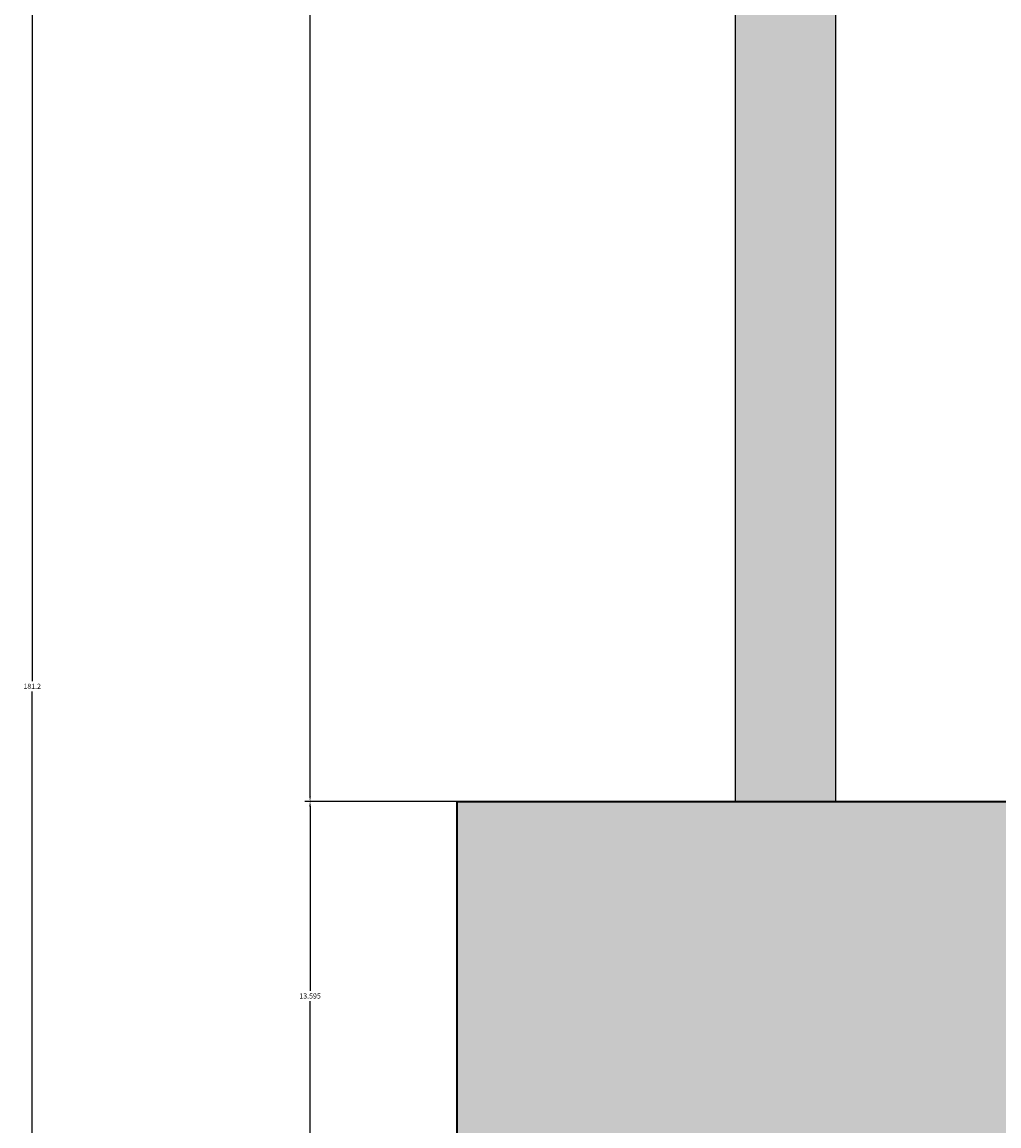
# Model space of a CAD drawing. Units: millimetres. Extents: x -11 to 280, y -4 to 208.
# Tile 6 of 55: x -10 to 24, y 87 to 125. Entities that reach past the tile are written whole.
import ezdxf

# ---------------------------------------------------------------- set-up
doc = ezdxf.new("R2010")
doc.units = ezdxf.units.MM
for name, color, linetype, lineweight in [('M-DIMS', 2, 'Continuous', 18), ('M-HYDR-EQPM', 7, 'Continuous', 35), ('M-HYDR-EQPM-PATT', 252, 'Continuous', 13), ('M-HYDR-RETN', 7, 'Continuous', 25)]:
    doc.layers.add(name, color=color, linetype=linetype, lineweight=lineweight)
doc.layers.add('M-HYDR-RETN-PATT', color=114, linetype='Continuous', lineweight=13, true_color=0x139b48)
doc.styles.get("Standard").update_dxf_attribs({"font": 'arial.ttf'})
doc.dimstyles.get("Standard").update_dxf_attribs({"dimtxt": 0.18, "dimasz": 0.18, "dimexe": 0.18, "dimexo": 0.0625, "dimgap": 0.09, "dimtad": 0, "dimtih": 1, "dimtoh": 1, "dimdec": 4, "dimzin": 0, "dimdsep": 46, "dimtxsty": 'Standard', "dimcen": 0.09, "dimadec": 0, "dimazin": 0, "dimtfac": 1, "dimtdec": 4, "dimtofl": 0, "dimtmove": 0, "dimatfit": 3, "dimfxl": 1, "dimtolj": 1, "dimtzin": 0, "dimarcsym": 0})

# ---------------------------------------------------------------- blocks, each defined once
blk = doc.blocks.new('*D5')
at = {"layer": 'Defpoints', "color": 0, "transparency": 16777216}
for p in [(24.759, 192.645), (-10.087, 11.435), (261.686, 11.435)]:
    blk.add_point(p, dxfattribs=at)
at = {"layer": 'M-DIMS', "color": 0, "lineweight": -2, "transparency": 16777216}
for p, q in [((24.696, 192.645), (-10.267, 192.645)), ((-10.087, 192.465), (-10.087, 102.222)), ((-10.087, 11.615), (-10.087, 101.858)), ((261.624, 11.435), (-10.267, 11.435))]:
    blk.add_line(p, q, dxfattribs=at)
at = {"layer": 'M-DIMS', "color": 0, "transparency": 16777216}
for points in [[(-10.117, 192.465), (-10.057, 192.465), (-10.087, 192.645)], [(-10.117, 11.615), (-10.057, 11.615), (-10.087, 11.435)]]:
    blk.add_solid(points, dxfattribs=at)
at = {"layer": 'M-DIMS', "color": 0, "transparency": 16777216, "insert": (-10.087, 102.04), "char_height": 0.18, "attachment_point": 5}
blk.add_mtext('\\A1;181.2', dxfattribs=at)
blk = doc.blocks.new('*D7')
at = {"layer": 'Defpoints', "color": 0, "transparency": 16777216}
for p in [(-0.38, 162.581), (14.47, 162.581), (14.47, 98.021)]:
    blk.add_point(p, dxfattribs=at)
at = {"layer": 'M-DIMS', "color": 0, "lineweight": -2, "transparency": 16777216}
for p, q in [((14.408, 162.581), (-0.56, 162.581)), ((-0.38, 162.401), (-0.38, 130.483)), ((-0.38, 98.201), (-0.38, 130.119)), ((14.408, 98.021), (-0.56, 98.021))]:
    blk.add_line(p, q, dxfattribs=at)
at = {"layer": 'M-DIMS', "color": 0, "transparency": 16777216}
for points in [[(-0.41, 162.401), (-0.35, 162.401), (-0.38, 162.581)], [(-0.41, 98.201), (-0.35, 98.201), (-0.38, 98.021)]]:
    blk.add_solid(points, dxfattribs=at)
at = {"layer": 'M-DIMS', "color": 0, "transparency": 16777216, "insert": (-0.38, 130.301), "char_height": 0.18, "attachment_point": 5}
blk.add_mtext('\\A1;64.56', dxfattribs=at)
blk = doc.blocks.new('*D28')
at = {"layer": 'Defpoints', "color": 0, "transparency": 16777216}
for p in [(-0.38, 98.021), (14.47, 98.021), (14.47, 84.426)]:
    blk.add_point(p, dxfattribs=at)
at = {"layer": 'M-DIMS', "color": 0, "lineweight": -2, "transparency": 16777216}
for p, q in [((14.408, 98.021), (-0.56, 98.021)), ((-0.38, 97.841), (-0.38, 91.406)), ((-0.38, 84.606), (-0.38, 91.042)), ((14.408, 84.426), (-0.56, 84.426))]:
    blk.add_line(p, q, dxfattribs=at)
at = {"layer": 'M-DIMS', "color": 0, "transparency": 16777216}
for points in [[(-0.41, 97.841), (-0.35, 97.841), (-0.38, 98.021)], [(-0.41, 84.606), (-0.35, 84.606), (-0.38, 84.426)]]:
    blk.add_solid(points, dxfattribs=at)
at = {"layer": 'M-DIMS', "color": 0, "transparency": 16777216, "insert": (-0.38, 91.224), "char_height": 0.18, "attachment_point": 5}
blk.add_mtext('\\A1;13.595', dxfattribs=at)

msp = doc.modelspace()

# ---------------------------------------------------------------- hatches: boundary and pattern name
at = {"layer": 'M-HYDR-EQPM-PATT'}
h = msp.add_hatch(color=256, dxfattribs=at)
h.set_gradient(color1=(69, 84, 165), color2=(0, 0, 255), tint=1)
h.paths.add_polyline_path([(31.0059, 84.4261), (31.0059, 98.0213), (4.7635, 98.0213), (4.7635, 84.4261)])
at = {"layer": 'M-HYDR-RETN-PATT'}
h = msp.add_hatch(color=256, dxfattribs=at)
h.set_gradient(color1=(19, 155, 72), color2=(19, 155, 72), tint=1)
h.paths.add_polyline_path([(17.9701, 159.0814), (29.2015, 159.0814), (29.2015, 162.5814), (14.4701, 162.5814), (14.4701, 98.0213), (17.9701, 98.0213)])
h.paths.add_polyline_path([(17.9701, 84.4261), (14.4701, 84.4261), (14.4701, 54.3099), (156.2446, 54.3099), (156.2446, 57.8099), (17.9701, 57.8099)])
h.paths.add_polyline_path([(120.5137, 74.3991), (17.9701, 74.3991), (17.9701, 70.8991), (120.5137, 70.8991)], flags=17)
h.paths.add_polyline_path([(184.7092, 75.04, 0.4142136), (179.7092, 80.04), (156.2446, 80.04), (156.2446, 57.8099), (156.2446, 54.3099), (156.2446, 43.5991), (159.7446, 43.5991), (159.7446, 57.8099), (159.7446, 76.54), (176.2092, 76.54, -0.4142136), (181.2092, 71.54), (181.2092, 57.8099), (159.7446, 57.8099), (159.7446, 54.3099), (184.7092, 54.3099)])

# ---------------------------------------------------------------- linework, layer by layer
at = {"layer": 'M-HYDR-EQPM'}
msp.add_lwpolyline([(4.7635, 98.0213), (31.0059, 98.0213), (31.0059, 84.4261), (4.7635, 84.4261)], close=True, dxfattribs=at)
at = {"layer": 'M-HYDR-RETN'}
for points in [[(14.4701, 162.5814), (14.4701, 98.0213)], [(17.9701, 159.0814), (17.9701, 98.0213)]]:
    msp.add_lwpolyline(points, dxfattribs=at)

# ---------------------------------------------------------------- dimensions: what is measured, and where the dimension line sits
at = {"layer": 'M-DIMS'}
for base, p1, p2, override, picture, middle in [((-10.0865, 11.4346), (24.7588, 192.645), (261.6863, 11.4346), {"dimdec": 1, "dimlfac": 1, "dimrnd": 0, "dimzin": 0, "dimdsep": 46, "dimlunit": 2}, '*D5', (-10.0865, 102.0398)), ((-0.3799, 162.5814), (14.4701, 98.0213), (14.4701, 162.5814), {"dimdec": 2, "dimlfac": 1, "dimrnd": 0, "dimzin": 0, "dimdsep": 46, "dimlunit": 2}, '*D7', (-0.3799, 130.3014)), ((-0.3799, 98.0213), (14.4701, 84.4261), (14.4701, 98.0213), {"dimdec": 3, "dimlfac": 1, "dimrnd": 0, "dimzin": 0, "dimdsep": 46, "dimlunit": 2}, '*D28', (-0.3799, 91.2237))]:
    dim = msp.add_linear_dim(base=base, p1=p1, p2=p2, angle=90, dimstyle='Standard', override=override, dxfattribs=at)
    dim.commit()
    dim.dimension.update_dxf_attribs({"geometry": picture, "text_midpoint": middle})

doc.saveas('drawing.dxf')
